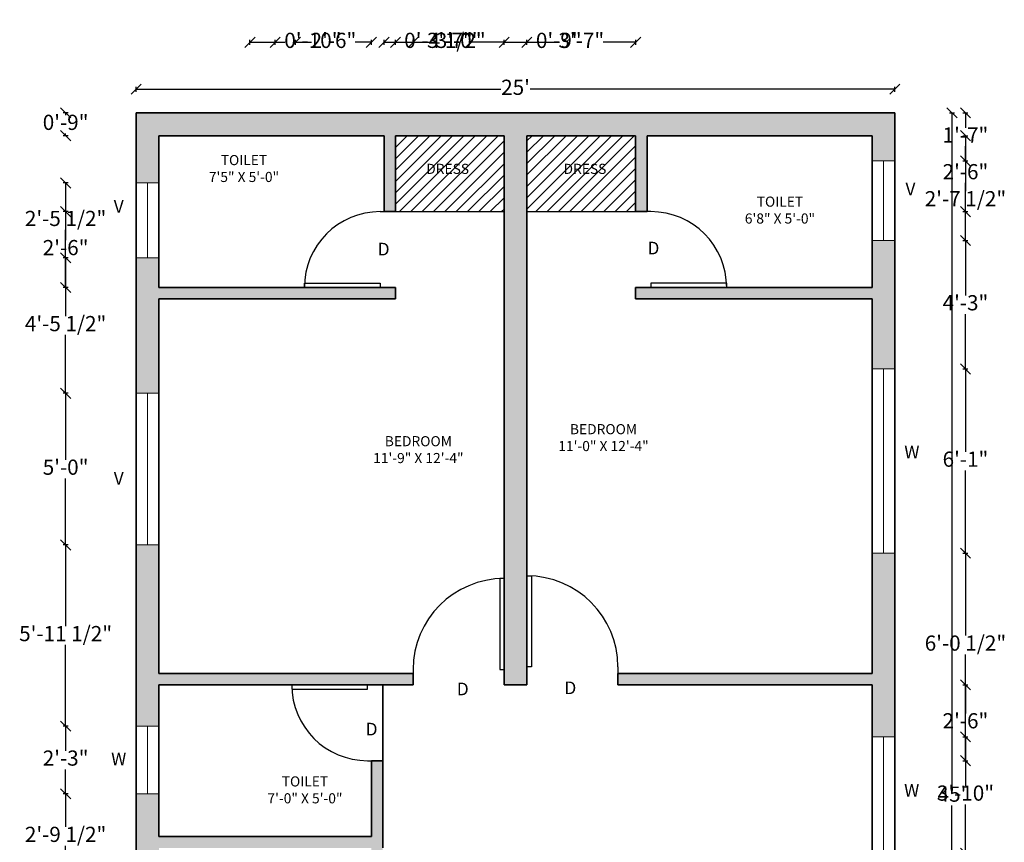
# Model space of a CAD drawing. Units: inches. Extents: x 2633 to 3023, y 679 to 1292.
# Tile 2 of 2: x 2633 to 3023, y 967 to 1292. Entities that reach past the tile are written whole.
import ezdxf

# ---------------------------------------------------------------- set-up
doc = ezdxf.new("R2010")
doc.units = ezdxf.units.IN
for name, color, linetype, lineweight in [('A-ANNO-DIMS', 2, 'Continuous', 18), ('A-ANNO-TEXT', 7, 'Continuous', 18), ('A-AREA-IDEN', 7, 'Continuous', 18), ('A-DOOR', 4, 'Continuous', 25), ('A-FURN', 8, 'Continuous', 25), ('A-FURN-PATT', 8, 'Continuous', 13), ('A-GLAZ', 1, 'Continuous', 18), ('A-WALL', 7, 'Continuous', 35), ('A-WALL-PATT', 5, 'Continuous', 13)]:
    doc.layers.add(name, color=color, linetype=linetype, lineweight=lineweight)
doc.styles.get("Standard").update_dxf_attribs({"font": 'arial.ttf'})
doc.dimstyles.new('ISO-25', dxfattribs={"dimtxt": 6, "dimasz": 4, "dimexe": 1, "dimexo": 1, "dimtad": 0, "dimtih": 1, "dimtoh": 1, "dimlunit": 3, "dimtxsty": 'Standard', "dimblk": 'OBLIQUE', "dimcen": 2.5, "dimadec": 0, "dimazin": 0, "dimtfac": 1, "dimtmove": 0, "dimatfit": 3, "dimfxl": 1, "dimfxlon": 1, "dimarcsym": 0})

# ---------------------------------------------------------------- blocks, each defined once
blk = doc.blocks.new('*U3')
for p, q in [((0, 0), (0, -6)), ((30, 0), (30, -6))]:
    blk.add_line(p, q)
blk.add_lwpolyline([(0, 0), (0, 30), (1.75, 30), (1.75, 0)], close=True)
blk.add_arc((0, 0), 30, 0, 90)
blk = doc.blocks.new('*U9')
for p, q in [((0, 0), (0, -6)), ((-36, 0), (-36, -6))]:
    blk.add_line(p, q)
blk.add_lwpolyline([(0, 0), (0, 36), (-1.75, 36), (-1.75, 0)], close=True)
blk.add_arc((0, 0), 36, 90, 180)
blk = doc.blocks.new('*U10')
for p, q in [((0, 0), (0, 6)), ((30, 0), (30, 6))]:
    blk.add_line(p, q)
blk.add_lwpolyline([(0, 0), (0, -30), (1.75, -30), (1.75, 0)], close=True)
blk.add_arc((0, 0), 30, 270, 0)
blk = doc.blocks.new('*U8')
for p, q in [((0, 0), (0, -6)), ((36, 0), (36, -6))]:
    blk.add_line(p, q)
blk.add_lwpolyline([(0, 0), (0, 36), (1.75, 36), (1.75, 0)], close=True)
blk.add_arc((0, 0), 36, 0, 90)
blk = doc.blocks.new('*U7')
for p, q in [((-30, 0), (-30, -6)), ((0, 0), (0, -6))]:
    blk.add_line(p, q)
blk.add_lwpolyline([(0, 0), (0, 30), (-1.75, 30), (-1.75, 0)], close=True)
blk.add_arc((0, 0), 30, 90, 180)
blk = doc.blocks.new('_Oblique')
at = {"color": 0, "linetype": 'ByBlock', "lineweight": -2}
blk.add_line((-0.5, -0.5), (0.5, 0.5), dxfattribs=at)
blk = doc.blocks.new('*D11')
at = {"layer": 'A-ANNO-DIMS', "color": 0, "lineweight": -2, "transparency": 16777216}
for p, q in [((2679.35, 1263.76), (2679.35, 1265.76)), ((2979.35, 1263.76), (2979.35, 1265.76)), ((2679.35, 1264.76), (2823.58, 1264.76)), ((2979.35, 1264.76), (2835.11, 1264.76))]:
    blk.add_line(p, q, dxfattribs=at)
at = {"layer": 'Defpoints', "color": 0, "transparency": 16777216}
for p in [(2979.35, 1264.76), (2679.35, 1255.4), (2979.35, 1255.4)]:
    blk.add_point(p, dxfattribs=at)
at = {"layer": 'A-ANNO-DIMS', "color": 0, "lineweight": -2, "transparency": 16777216, "xscale": 4, "yscale": 4, "zscale": 4, "rotation": 180}
blk.add_blockref('_Oblique', (2679.35, 1264.76), dxfattribs=at)
at = {"layer": 'A-ANNO-DIMS', "color": 0, "lineweight": -2, "transparency": 16777216, "xscale": 4, "yscale": 4, "zscale": 4}
blk.add_blockref('_Oblique', (2979.35, 1264.76), dxfattribs=at)
at = {"layer": 'A-ANNO-DIMS', "color": 0, "transparency": 16777216, "insert": (2829.35, 1264.76), "char_height": 6, "attachment_point": 5}
blk.add_mtext("25'", dxfattribs=at)
blk = doc.blocks.new('*D12')
at = {"layer": 'A-ANNO-DIMS', "color": 0, "lineweight": -2, "transparency": 16777216}
for p, q in [((3000.92, 1255.4), (3002.92, 1255.4)), ((3001.92, 1255.4), (3001.92, 989.07)), ((3001.92, 715.4), (3001.92, 981.72)), ((3000.92, 715.4), (3002.92, 715.4))]:
    blk.add_line(p, q, dxfattribs=at)
at = {"layer": 'Defpoints', "color": 0, "transparency": 16777216}
for p in [(2979.35, 1255.4), (2979.35, 715.4), (3001.92, 715.4)]:
    blk.add_point(p, dxfattribs=at)
at = {"layer": 'A-ANNO-DIMS', "color": 0, "lineweight": -2, "transparency": 16777216, "xscale": 4, "yscale": 4, "zscale": 4}
for p, rotation in [((3001.92, 1255.4), 90), ((3001.92, 715.4), 270)]:
    blk.add_blockref('_Oblique', p, dxfattribs=dict(at, rotation=rotation))
at = {"layer": 'A-ANNO-DIMS', "color": 0, "transparency": 16777216, "insert": (3001.92, 985.4), "char_height": 6, "attachment_point": 5}
blk.add_mtext("45'", dxfattribs=at)
blk = doc.blocks.new('*D13')
at = {"layer": 'A-ANNO-DIMS', "color": 0, "lineweight": -2, "transparency": 16777216}
for p, q in [((2777.35, 1282.3), (2777.35, 1284.3)), ((2777.35, 1283.3), (2781.85, 1283.3)), ((2781.85, 1282.3), (2781.85, 1284.3)), ((2781.85, 1283.3), (2785.85, 1283.3))]:
    blk.add_line(p, q, dxfattribs=at)
at = {"layer": 'Defpoints', "color": 0, "transparency": 16777216}
for p in [(2781.85, 1283.3), (2777.35, 1246.4), (2781.85, 1246.4)]:
    blk.add_point(p, dxfattribs=at)
at = {"layer": 'A-ANNO-DIMS', "color": 0, "lineweight": -2, "transparency": 16777216, "xscale": 4, "yscale": 4, "zscale": 4, "rotation": 180}
blk.add_blockref('_Oblique', (2777.35, 1283.3), dxfattribs=at)
at = {"layer": 'A-ANNO-DIMS', "color": 0, "lineweight": -2, "transparency": 16777216, "xscale": 4, "yscale": 4, "zscale": 4}
blk.add_blockref('_Oblique', (2781.85, 1283.3), dxfattribs=at)
at = {"layer": 'A-ANNO-DIMS', "color": 0, "transparency": 16777216, "insert": (2801.44, 1283.3), "char_height": 6, "attachment_point": 5}
blk.add_mtext('0\'-4 1/2"', dxfattribs=at)
blk = doc.blocks.new('*D14')
at = {"layer": 'A-ANNO-DIMS', "color": 0, "lineweight": -2, "transparency": 16777216}
for p, q in [((2781.85, 1282.3), (2781.85, 1284.3)), ((2781.85, 1283.3), (2794.75, 1283.3)), ((2824.85, 1283.3), (2811.94, 1283.3)), ((2824.85, 1282.3), (2824.85, 1284.3))]:
    blk.add_line(p, q, dxfattribs=at)
at = {"layer": 'Defpoints', "color": 0, "transparency": 16777216}
for p in [(2824.85, 1283.3), (2781.85, 1246.4), (2824.85, 1246.4)]:
    blk.add_point(p, dxfattribs=at)
at = {"layer": 'A-ANNO-DIMS', "color": 0, "lineweight": -2, "transparency": 16777216, "xscale": 4, "yscale": 4, "zscale": 4, "rotation": 180}
blk.add_blockref('_Oblique', (2781.85, 1283.3), dxfattribs=at)
at = {"layer": 'A-ANNO-DIMS', "color": 0, "lineweight": -2, "transparency": 16777216, "xscale": 4, "yscale": 4, "zscale": 4}
blk.add_blockref('_Oblique', (2824.85, 1283.3), dxfattribs=at)
at = {"layer": 'A-ANNO-DIMS', "color": 0, "transparency": 16777216, "insert": (2803.35, 1283.3), "char_height": 6, "attachment_point": 5}
blk.add_mtext('3\'-7"', dxfattribs=at)
blk = doc.blocks.new('*D15')
at = {"layer": 'A-ANNO-DIMS', "color": 0, "lineweight": -2, "transparency": 16777216}
for p, q in [((2824.85, 1282.3), (2824.85, 1284.3)), ((2824.85, 1283.3), (2833.85, 1283.3)), ((2833.85, 1282.3), (2833.85, 1284.3)), ((2833.85, 1283.3), (2837.85, 1283.3))]:
    blk.add_line(p, q, dxfattribs=at)
at = {"layer": 'Defpoints', "color": 0, "transparency": 16777216}
for p in [(2833.85, 1283.3), (2824.85, 1246.4), (2833.85, 1246.4)]:
    blk.add_point(p, dxfattribs=at)
at = {"layer": 'A-ANNO-DIMS', "color": 0, "lineweight": -2, "transparency": 16777216, "xscale": 4, "yscale": 4, "zscale": 4, "rotation": 180}
blk.add_blockref('_Oblique', (2824.85, 1283.3), dxfattribs=at)
at = {"layer": 'A-ANNO-DIMS', "color": 0, "lineweight": -2, "transparency": 16777216, "xscale": 4, "yscale": 4, "zscale": 4}
blk.add_blockref('_Oblique', (2833.85, 1283.3), dxfattribs=at)
at = {"layer": 'A-ANNO-DIMS', "color": 0, "transparency": 16777216, "insert": (2846.45, 1283.3), "char_height": 6, "attachment_point": 5}
blk.add_mtext('0\'-9"', dxfattribs=at)
blk = doc.blocks.new('*D16')
at = {"layer": 'A-ANNO-DIMS', "color": 0, "lineweight": -2, "transparency": 16777216}
for p, q in [((3006.25, 1246.4), (3008.25, 1246.4)), ((3007.25, 1246.4), (3007.25, 1235.08)), ((3007.25, 1216.4), (3007.25, 1227.71)), ((3006.25, 1216.4), (3008.25, 1216.4))]:
    blk.add_line(p, q, dxfattribs=at)
at = {"layer": 'Defpoints', "color": 0, "transparency": 16777216}
for p in [(2833.85, 1246.4), (3007.25, 1246.4), (2833.85, 1216.4)]:
    blk.add_point(p, dxfattribs=at)
at = {"layer": 'A-ANNO-DIMS', "color": 0, "lineweight": -2, "transparency": 16777216, "xscale": 4, "yscale": 4, "zscale": 4}
for p, rotation in [((3007.25, 1246.4), 90), ((3007.25, 1216.4), 270)]:
    blk.add_blockref('_Oblique', p, dxfattribs=dict(at, rotation=rotation))
at = {"layer": 'A-ANNO-DIMS', "color": 0, "transparency": 16777216, "insert": (3007.25, 1231.4), "char_height": 6, "attachment_point": 5}
blk.add_mtext('2\'-6"', dxfattribs=at)
blk = doc.blocks.new('*D17')
at = {"layer": 'A-ANNO-DIMS', "color": 0, "lineweight": -2, "transparency": 16777216}
for p, q in [((2833.85, 1282.3), (2833.85, 1284.3)), ((2833.85, 1283.3), (2846.75, 1283.3)), ((2876.85, 1283.3), (2863.94, 1283.3)), ((2876.85, 1282.3), (2876.85, 1284.3))]:
    blk.add_line(p, q, dxfattribs=at)
at = {"layer": 'Defpoints', "color": 0, "transparency": 16777216}
for p in [(2876.85, 1283.3), (2833.85, 1246.4), (2876.85, 1246.4)]:
    blk.add_point(p, dxfattribs=at)
at = {"layer": 'A-ANNO-DIMS', "color": 0, "lineweight": -2, "transparency": 16777216, "xscale": 4, "yscale": 4, "zscale": 4, "rotation": 180}
blk.add_blockref('_Oblique', (2833.85, 1283.3), dxfattribs=at)
at = {"layer": 'A-ANNO-DIMS', "color": 0, "lineweight": -2, "transparency": 16777216, "xscale": 4, "yscale": 4, "zscale": 4}
blk.add_blockref('_Oblique', (2876.85, 1283.3), dxfattribs=at)
at = {"layer": 'A-ANNO-DIMS', "color": 0, "transparency": 16777216, "insert": (2855.35, 1283.3), "char_height": 6, "attachment_point": 5}
blk.add_mtext('3\'-7"', dxfattribs=at)
blk = doc.blocks.new('*D20')
at = {"layer": 'A-ANNO-DIMS', "color": 0, "lineweight": -2, "transparency": 16777216}
for p, q in [((2724.35, 1282.3), (2724.35, 1284.3)), ((2724.35, 1283.3), (2734.3, 1283.3)), ((2734.3, 1282.3), (2734.3, 1284.3)), ((2734.3, 1283.3), (2738.3, 1283.3))]:
    blk.add_line(p, q, dxfattribs=at)
at = {"layer": 'Defpoints', "color": 0, "transparency": 16777216}
for p in [(2734.3, 1283.3), (2724.35, 724.4), (2734.3, 724.4)]:
    blk.add_point(p, dxfattribs=at)
at = {"layer": 'A-ANNO-DIMS', "color": 0, "lineweight": -2, "transparency": 16777216, "xscale": 4, "yscale": 4, "zscale": 4, "rotation": 180}
blk.add_blockref('_Oblique', (2724.35, 1283.3), dxfattribs=at)
at = {"layer": 'A-ANNO-DIMS', "color": 0, "lineweight": -2, "transparency": 16777216, "xscale": 4, "yscale": 4, "zscale": 4}
blk.add_blockref('_Oblique', (2734.3, 1283.3), dxfattribs=at)
at = {"layer": 'A-ANNO-DIMS', "color": 0, "transparency": 16777216, "insert": (2749.23, 1283.3), "char_height": 6, "attachment_point": 5}
blk.add_mtext('0\'-10"', dxfattribs=at)
blk = doc.blocks.new('*D23')
at = {"layer": 'A-ANNO-DIMS', "color": 0, "lineweight": -2, "transparency": 16777216}
for p, q in [((2788.85, 1282.3), (2788.85, 1284.3)), ((2788.85, 1283.3), (2798.25, 1283.3)), ((2824.85, 1283.3), (2815.44, 1283.3)), ((2824.85, 1282.3), (2824.85, 1284.3))]:
    blk.add_line(p, q, dxfattribs=at)
at = {"layer": 'Defpoints', "color": 0, "transparency": 16777216}
for p in [(2824.85, 1283.3), (2788.85, 1033.9), (2824.85, 1033.65)]:
    blk.add_point(p, dxfattribs=at)
at = {"layer": 'A-ANNO-DIMS', "color": 0, "lineweight": -2, "transparency": 16777216, "xscale": 4, "yscale": 4, "zscale": 4, "rotation": 180}
blk.add_blockref('_Oblique', (2788.85, 1283.3), dxfattribs=at)
at = {"layer": 'A-ANNO-DIMS', "color": 0, "lineweight": -2, "transparency": 16777216, "xscale": 4, "yscale": 4, "zscale": 4}
blk.add_blockref('_Oblique', (2824.85, 1283.3), dxfattribs=at)
at = {"layer": 'A-ANNO-DIMS', "color": 0, "transparency": 16777216, "insert": (2806.85, 1283.3), "char_height": 6, "attachment_point": 5}
blk.add_mtext('3\'-0"', dxfattribs=at)
blk = doc.blocks.new('*D25')
at = {"layer": 'A-ANNO-DIMS', "color": 0, "lineweight": -2, "transparency": 16777216}
for p, q in [((2742.35, 1282.3), (2742.35, 1284.3)), ((2742.35, 1283.3), (2748.7, 1283.3)), ((2772.35, 1283.3), (2766, 1283.3)), ((2772.35, 1282.3), (2772.35, 1284.3))]:
    blk.add_line(p, q, dxfattribs=at)
at = {"layer": 'Defpoints', "color": 0, "transparency": 16777216}
for p in [(2772.35, 1283.3), (2742.35, 904.9), (2772.35, 904.65)]:
    blk.add_point(p, dxfattribs=at)
at = {"layer": 'A-ANNO-DIMS', "color": 0, "lineweight": -2, "transparency": 16777216, "xscale": 4, "yscale": 4, "zscale": 4, "rotation": 180}
blk.add_blockref('_Oblique', (2742.35, 1283.3), dxfattribs=at)
at = {"layer": 'A-ANNO-DIMS', "color": 0, "lineweight": -2, "transparency": 16777216, "xscale": 4, "yscale": 4, "zscale": 4}
blk.add_blockref('_Oblique', (2772.35, 1283.3), dxfattribs=at)
at = {"layer": 'A-ANNO-DIMS', "color": 0, "transparency": 16777216, "insert": (2757.35, 1283.3), "char_height": 6, "attachment_point": 5}
blk.add_mtext('2\'-6"', dxfattribs=at)
blk = doc.blocks.new('*D26')
at = {"layer": 'A-ANNO-DIMS', "color": 0, "lineweight": -2, "transparency": 16777216}
for p, q in [((2652.45, 1216.4), (2650.45, 1216.4)), ((2651.45, 1216.4), (2651.45, 1205.08)), ((2651.45, 1186.4), (2651.45, 1197.71)), ((2652.45, 1186.4), (2650.45, 1186.4))]:
    blk.add_line(p, q, dxfattribs=at)
at = {"layer": 'Defpoints', "color": 0, "transparency": 16777216}
for p in [(2777.35, 1216.4), (2651.45, 1186.4), (2777.6, 1186.4)]:
    blk.add_point(p, dxfattribs=at)
at = {"layer": 'A-ANNO-DIMS', "color": 0, "lineweight": -2, "transparency": 16777216, "xscale": 4, "yscale": 4, "zscale": 4}
for p, rotation in [((2651.45, 1216.4), 90), ((2651.45, 1186.4), 270)]:
    blk.add_blockref('_Oblique', p, dxfattribs=dict(at, rotation=rotation))
at = {"layer": 'A-ANNO-DIMS', "color": 0, "transparency": 16777216, "insert": (2651.45, 1201.4), "char_height": 6, "attachment_point": 5}
blk.add_mtext('2\'-6"', dxfattribs=at)
blk = doc.blocks.new('*D27')
at = {"layer": 'A-ANNO-DIMS', "color": 0, "lineweight": -2, "transparency": 16777216}
for p, q in [((3006.25, 1029.4), (3008.25, 1029.4)), ((3007.25, 1029.4), (3007.25, 1018.08)), ((3007.25, 999.4), (3007.25, 1010.71)), ((3006.25, 999.4), (3008.25, 999.4))]:
    blk.add_line(p, q, dxfattribs=at)
at = {"layer": 'Defpoints', "color": 0, "transparency": 16777216}
for p in [(2776.85, 1029.4), (3007.25, 1029.4), (2776.85, 999.4)]:
    blk.add_point(p, dxfattribs=at)
at = {"layer": 'A-ANNO-DIMS', "color": 0, "lineweight": -2, "transparency": 16777216, "xscale": 4, "yscale": 4, "zscale": 4}
for p, rotation in [((3007.25, 1029.4), 90), ((3007.25, 999.4), 270)]:
    blk.add_blockref('_Oblique', p, dxfattribs=dict(at, rotation=rotation))
at = {"layer": 'A-ANNO-DIMS', "color": 0, "transparency": 16777216, "insert": (3007.25, 1014.4), "char_height": 6, "attachment_point": 5}
blk.add_mtext('2\'-6"', dxfattribs=at)
blk = doc.blocks.new('*D28')
at = {"layer": 'A-ANNO-DIMS', "color": 0, "lineweight": -2, "transparency": 16777216}
for p, q in [((2652.45, 1255.4), (2650.45, 1255.4)), ((2651.45, 1255.4), (2651.45, 1254.58)), ((2652.45, 1246.4), (2650.45, 1246.4)), ((2651.45, 1246.4), (2651.45, 1247.21))]:
    blk.add_line(p, q, dxfattribs=at)
at = {"layer": 'Defpoints', "color": 0, "transparency": 16777216}
for p in [(2679.35, 1255.4), (2651.45, 1246.4), (2688.35, 1246.4)]:
    blk.add_point(p, dxfattribs=at)
at = {"layer": 'A-ANNO-DIMS', "color": 0, "lineweight": -2, "transparency": 16777216, "xscale": 4, "yscale": 4, "zscale": 4}
for p, rotation in [((2651.45, 1255.4), 90), ((2651.45, 1246.4), 270)]:
    blk.add_blockref('_Oblique', p, dxfattribs=dict(at, rotation=rotation))
at = {"layer": 'A-ANNO-DIMS', "color": 0, "transparency": 16777216, "insert": (2651.45, 1250.9), "char_height": 6, "attachment_point": 5}
blk.add_mtext('0\'-9"', dxfattribs=at)
blk = doc.blocks.new('*D33')
at = {"layer": 'A-ANNO-DIMS', "color": 0, "lineweight": -2, "transparency": 16777216}
for p, q in [((2652.45, 986.26), (2650.45, 986.26)), ((2651.45, 986.26), (2651.45, 973.23)), ((2651.45, 952.74), (2651.45, 965.77)), ((2652.45, 952.74), (2650.45, 952.74))]:
    blk.add_line(p, q, dxfattribs=at)
at = {"layer": 'Defpoints', "color": 0, "transparency": 16777216}
for p in [(2651.45, 986.26), (2679.35, 986.26), (2679.35, 952.74)]:
    blk.add_point(p, dxfattribs=at)
at = {"layer": 'A-ANNO-DIMS', "color": 0, "lineweight": -2, "transparency": 16777216, "xscale": 4, "yscale": 4, "zscale": 4}
for p, rotation in [((2651.45, 986.26), 90), ((2651.45, 952.74), 270)]:
    blk.add_blockref('_Oblique', p, dxfattribs=dict(at, rotation=rotation))
at = {"layer": 'A-ANNO-DIMS', "color": 0, "transparency": 16777216, "insert": (2651.45, 969.5), "char_height": 6, "attachment_point": 5}
blk.add_mtext('2\'-9 1/2"', dxfattribs=at)
blk = doc.blocks.new('*D34')
at = {"layer": 'A-ANNO-DIMS', "color": 0, "lineweight": -2, "transparency": 16777216}
for p, q in [((2652.45, 1013.04), (2650.45, 1013.04)), ((2651.45, 1013.04), (2651.45, 1003.34)), ((2651.45, 986.26), (2651.45, 995.96)), ((2652.45, 986.26), (2650.45, 986.26))]:
    blk.add_line(p, q, dxfattribs=at)
at = {"layer": 'Defpoints', "color": 0, "transparency": 16777216}
for p in [(2651.45, 1013.04), (2679.35, 1013.04), (2679.35, 986.26)]:
    blk.add_point(p, dxfattribs=at)
at = {"layer": 'A-ANNO-DIMS', "color": 0, "lineweight": -2, "transparency": 16777216, "xscale": 4, "yscale": 4, "zscale": 4}
for p, rotation in [((2651.45, 1013.04), 90), ((2651.45, 986.26), 270)]:
    blk.add_blockref('_Oblique', p, dxfattribs=dict(at, rotation=rotation))
at = {"layer": 'A-ANNO-DIMS', "color": 0, "transparency": 16777216, "insert": (2651.45, 999.65), "char_height": 6, "attachment_point": 5}
blk.add_mtext('2\'-3"', dxfattribs=at)
blk = doc.blocks.new('*D35')
at = {"layer": 'A-ANNO-DIMS', "color": 0, "lineweight": -2, "transparency": 16777216}
for p, q in [((2652.45, 1084.66), (2650.45, 1084.66)), ((2651.45, 1084.66), (2651.45, 1052.58)), ((2651.45, 1013.04), (2651.45, 1045.12)), ((2652.45, 1013.04), (2650.45, 1013.04))]:
    blk.add_line(p, q, dxfattribs=at)
at = {"layer": 'Defpoints', "color": 0, "transparency": 16777216}
for p in [(2651.45, 1084.66), (2679.35, 1084.66), (2679.35, 1013.04)]:
    blk.add_point(p, dxfattribs=at)
at = {"layer": 'A-ANNO-DIMS', "color": 0, "lineweight": -2, "transparency": 16777216, "xscale": 4, "yscale": 4, "zscale": 4}
for p, rotation in [((2651.45, 1084.66), 90), ((2651.45, 1013.04), 270)]:
    blk.add_blockref('_Oblique', p, dxfattribs=dict(at, rotation=rotation))
at = {"layer": 'A-ANNO-DIMS', "color": 0, "transparency": 16777216, "insert": (2651.45, 1048.85), "char_height": 6, "attachment_point": 5}
blk.add_mtext('5\'-11 1/2"', dxfattribs=at)
blk = doc.blocks.new('*D36')
at = {"layer": 'A-ANNO-DIMS', "color": 0, "lineweight": -2, "transparency": 16777216}
for p, q in [((2652.45, 1144.59), (2650.45, 1144.59)), ((2651.45, 1144.59), (2651.45, 1118.31)), ((2651.45, 1084.66), (2651.45, 1110.94)), ((2652.45, 1084.66), (2650.45, 1084.66))]:
    blk.add_line(p, q, dxfattribs=at)
at = {"layer": 'Defpoints', "color": 0, "transparency": 16777216}
for p in [(2651.45, 1144.59), (2679.35, 1144.59), (2679.35, 1084.66)]:
    blk.add_point(p, dxfattribs=at)
at = {"layer": 'A-ANNO-DIMS', "color": 0, "lineweight": -2, "transparency": 16777216, "xscale": 4, "yscale": 4, "zscale": 4}
for p, rotation in [((2651.45, 1144.59), 90), ((2651.45, 1084.66), 270)]:
    blk.add_blockref('_Oblique', p, dxfattribs=dict(at, rotation=rotation))
at = {"layer": 'A-ANNO-DIMS', "color": 0, "transparency": 16777216, "insert": (2651.45, 1114.62), "char_height": 6, "attachment_point": 5}
blk.add_mtext('5\'-0"', dxfattribs=at)
blk = doc.blocks.new('*D37')
at = {"layer": 'A-ANNO-DIMS', "color": 0, "lineweight": -2, "transparency": 16777216}
for p, q in [((2652.45, 1198.14), (2650.45, 1198.14)), ((2651.45, 1198.14), (2651.45, 1175.09)), ((2651.45, 1144.59), (2651.45, 1167.64)), ((2652.45, 1144.59), (2650.45, 1144.59))]:
    blk.add_line(p, q, dxfattribs=at)
at = {"layer": 'Defpoints', "color": 0, "transparency": 16777216}
for p in [(2651.45, 1198.14), (2679.35, 1198.14), (2679.35, 1144.59)]:
    blk.add_point(p, dxfattribs=at)
at = {"layer": 'A-ANNO-DIMS', "color": 0, "lineweight": -2, "transparency": 16777216, "xscale": 4, "yscale": 4, "zscale": 4}
for p, rotation in [((2651.45, 1198.14), 90), ((2651.45, 1144.59), 270)]:
    blk.add_blockref('_Oblique', p, dxfattribs=dict(at, rotation=rotation))
at = {"layer": 'A-ANNO-DIMS', "color": 0, "transparency": 16777216, "insert": (2651.45, 1171.36), "char_height": 6, "attachment_point": 5}
blk.add_mtext('4\'-5 1/2"', dxfattribs=at)
blk = doc.blocks.new('*D38')
at = {"layer": 'A-ANNO-DIMS', "color": 0, "lineweight": -2, "transparency": 16777216}
for p, q in [((2652.45, 1227.71), (2650.45, 1227.71)), ((2651.45, 1227.71), (2651.45, 1216.65)), ((2651.45, 1198.14), (2651.45, 1209.2)), ((2652.45, 1198.14), (2650.45, 1198.14))]:
    blk.add_line(p, q, dxfattribs=at)
at = {"layer": 'Defpoints', "color": 0, "transparency": 16777216}
for p in [(2651.45, 1227.71), (2679.35, 1227.71), (2679.35, 1198.14)]:
    blk.add_point(p, dxfattribs=at)
at = {"layer": 'A-ANNO-DIMS', "color": 0, "lineweight": -2, "transparency": 16777216, "xscale": 4, "yscale": 4, "zscale": 4}
for p, rotation in [((2651.45, 1227.71), 90), ((2651.45, 1198.14), 270)]:
    blk.add_blockref('_Oblique', p, dxfattribs=dict(at, rotation=rotation))
at = {"layer": 'A-ANNO-DIMS', "color": 0, "transparency": 16777216, "insert": (2651.45, 1212.92), "char_height": 6, "attachment_point": 5}
blk.add_mtext('2\'-5 1/2"', dxfattribs=at)
blk = doc.blocks.new('*D42')
at = {"layer": 'A-ANNO-DIMS', "color": 0, "lineweight": -2, "transparency": 16777216}
for p, q in [((3006.25, 1008.83), (3008.25, 1008.83)), ((3007.25, 1008.83), (3007.25, 989.5)), ((3007.25, 962.79), (3007.25, 982.12)), ((3006.25, 962.79), (3008.25, 962.79))]:
    blk.add_line(p, q, dxfattribs=at)
at = {"layer": 'Defpoints', "color": 0, "transparency": 16777216}
for p in [(2979.35, 1008.83), (3007.25, 1008.83), (2979.35, 962.79)]:
    blk.add_point(p, dxfattribs=at)
at = {"layer": 'A-ANNO-DIMS', "color": 0, "lineweight": -2, "transparency": 16777216, "xscale": 4, "yscale": 4, "zscale": 4}
for p, rotation in [((3007.25, 1008.83), 90), ((3007.25, 962.79), 270)]:
    blk.add_blockref('_Oblique', p, dxfattribs=dict(at, rotation=rotation))
at = {"layer": 'A-ANNO-DIMS', "color": 0, "transparency": 16777216, "insert": (3007.25, 985.81), "char_height": 6, "attachment_point": 5}
blk.add_mtext('3\'-10"', dxfattribs=at)
blk = doc.blocks.new('*D43')
at = {"layer": 'A-ANNO-DIMS', "color": 0, "lineweight": -2, "transparency": 16777216}
for p, q in [((3006.25, 1081.38), (3008.25, 1081.38)), ((3007.25, 1081.38), (3007.25, 1048.83)), ((3007.25, 1008.83), (3007.25, 1041.38)), ((3006.25, 1008.83), (3008.25, 1008.83))]:
    blk.add_line(p, q, dxfattribs=at)
at = {"layer": 'Defpoints', "color": 0, "transparency": 16777216}
for p in [(2979.35, 1081.38), (3007.25, 1081.38), (2979.35, 1008.83)]:
    blk.add_point(p, dxfattribs=at)
at = {"layer": 'A-ANNO-DIMS', "color": 0, "lineweight": -2, "transparency": 16777216, "xscale": 4, "yscale": 4, "zscale": 4}
for p, rotation in [((3007.25, 1081.38), 90), ((3007.25, 1008.83), 270)]:
    blk.add_blockref('_Oblique', p, dxfattribs=dict(at, rotation=rotation))
at = {"layer": 'A-ANNO-DIMS', "color": 0, "transparency": 16777216, "insert": (3007.25, 1045.1), "char_height": 6, "attachment_point": 5}
blk.add_mtext('6\'-0 1/2"', dxfattribs=at)
blk = doc.blocks.new('*D44')
at = {"layer": 'A-ANNO-DIMS', "color": 0, "lineweight": -2, "transparency": 16777216}
for p, q in [((3006.25, 1154.2), (3008.25, 1154.2)), ((3007.25, 1154.2), (3007.25, 1121.48)), ((3007.25, 1081.38), (3007.25, 1114.1)), ((3006.25, 1081.38), (3008.25, 1081.38))]:
    blk.add_line(p, q, dxfattribs=at)
at = {"layer": 'Defpoints', "color": 0, "transparency": 16777216}
for p in [(2979.35, 1154.2), (3007.25, 1154.2), (2979.35, 1081.38)]:
    blk.add_point(p, dxfattribs=at)
at = {"layer": 'A-ANNO-DIMS', "color": 0, "lineweight": -2, "transparency": 16777216, "xscale": 4, "yscale": 4, "zscale": 4}
for p, rotation in [((3007.25, 1154.2), 90), ((3007.25, 1081.38), 270)]:
    blk.add_blockref('_Oblique', p, dxfattribs=dict(at, rotation=rotation))
at = {"layer": 'A-ANNO-DIMS', "color": 0, "transparency": 16777216, "insert": (3007.25, 1117.79), "char_height": 6, "attachment_point": 5}
blk.add_mtext('6\'-1"', dxfattribs=at)
blk = doc.blocks.new('*D45')
at = {"layer": 'A-ANNO-DIMS', "color": 0, "lineweight": -2, "transparency": 16777216}
for p, q in [((3006.25, 1205.01), (3008.25, 1205.01)), ((3007.25, 1205.01), (3007.25, 1183.29)), ((3007.25, 1154.2), (3007.25, 1175.91)), ((3006.25, 1154.2), (3008.25, 1154.2))]:
    blk.add_line(p, q, dxfattribs=at)
at = {"layer": 'Defpoints', "color": 0, "transparency": 16777216}
for p in [(2979.35, 1205.01), (3007.25, 1205.01), (2979.35, 1154.2)]:
    blk.add_point(p, dxfattribs=at)
at = {"layer": 'A-ANNO-DIMS', "color": 0, "lineweight": -2, "transparency": 16777216, "xscale": 4, "yscale": 4, "zscale": 4}
for p, rotation in [((3007.25, 1205.01), 90), ((3007.25, 1154.2), 270)]:
    blk.add_blockref('_Oblique', p, dxfattribs=dict(at, rotation=rotation))
at = {"layer": 'A-ANNO-DIMS', "color": 0, "transparency": 16777216, "insert": (3007.25, 1179.6), "char_height": 6, "attachment_point": 5}
blk.add_mtext('4\'-3"', dxfattribs=at)
blk = doc.blocks.new('*D46')
at = {"layer": 'A-ANNO-DIMS', "color": 0, "lineweight": -2, "transparency": 16777216}
for p, q in [((3006.25, 1236.41), (3008.25, 1236.41)), ((3007.25, 1236.41), (3007.25, 1224.44)), ((3007.25, 1205.01), (3007.25, 1216.98)), ((3006.25, 1205.01), (3008.25, 1205.01))]:
    blk.add_line(p, q, dxfattribs=at)
at = {"layer": 'Defpoints', "color": 0, "transparency": 16777216}
for p in [(2979.35, 1236.41), (3007.25, 1236.41), (2979.35, 1205.01)]:
    blk.add_point(p, dxfattribs=at)
at = {"layer": 'A-ANNO-DIMS', "color": 0, "lineweight": -2, "transparency": 16777216, "xscale": 4, "yscale": 4, "zscale": 4}
for p, rotation in [((3007.25, 1236.41), 90), ((3007.25, 1205.01), 270)]:
    blk.add_blockref('_Oblique', p, dxfattribs=dict(at, rotation=rotation))
at = {"layer": 'A-ANNO-DIMS', "color": 0, "transparency": 16777216, "insert": (3007.25, 1220.71), "char_height": 6, "attachment_point": 5}
blk.add_mtext('2\'-7 1/2"', dxfattribs=at)
blk = doc.blocks.new('*D47')
at = {"layer": 'A-ANNO-DIMS', "color": 0, "lineweight": -2, "transparency": 16777216}
for p, q in [((3006.25, 1255.4), (3008.25, 1255.4)), ((3007.25, 1255.4), (3007.25, 1249.54)), ((3007.25, 1236.41), (3007.25, 1242.27)), ((3006.25, 1236.41), (3008.25, 1236.41))]:
    blk.add_line(p, q, dxfattribs=at)
at = {"layer": 'Defpoints', "color": 0, "transparency": 16777216}
for p in [(2979.35, 1255.4), (3007.25, 1255.4), (2979.35, 1236.41)]:
    blk.add_point(p, dxfattribs=at)
at = {"layer": 'A-ANNO-DIMS', "color": 0, "lineweight": -2, "transparency": 16777216, "xscale": 4, "yscale": 4, "zscale": 4}
for p, rotation in [((3007.25, 1255.4), 90), ((3007.25, 1236.41), 270)]:
    blk.add_blockref('_Oblique', p, dxfattribs=dict(at, rotation=rotation))
at = {"layer": 'A-ANNO-DIMS', "color": 0, "transparency": 16777216, "insert": (3007.25, 1245.9), "char_height": 6, "attachment_point": 5}
blk.add_mtext('1\'-7"', dxfattribs=at)

msp = doc.modelspace()

# ---------------------------------------------------------------- hatches: boundary and pattern name
at = {"layer": 'A-FURN-PATT'}
h = msp.add_hatch(dxfattribs=at)
h.set_pattern_fill('ANSI31', color=256)
h.paths.add_polyline_path([(2824.847, 1246.396), (2781.847, 1246.396), (2781.847, 1216.396), (2824.847, 1216.396)])
h.paths.add_polyline_path([(2876.847, 1246.396), (2833.847, 1246.396), (2833.847, 1216.396), (2876.847, 1216.396)])
h.paths.add_polyline_path([(2791.81, 1229.045), (2813.063, 1229.045), (2813.063, 1237.288), (2791.81, 1237.288)], flags=24)
h.paths.add_polyline_path([(2846.101, 1229.045), (2867.354, 1229.045), (2867.354, 1237.288), (2846.101, 1237.288)], flags=24)
at = {"layer": 'A-WALL-PATT'}
h = msp.add_hatch(color=256, dxfattribs=at)
h.dxf.hatch_style = 1
h.paths.add_polyline_path([(2777.347, 1246.396), (2777.347, 1216.396), (2781.847, 1216.396), (2781.847, 1246.396), (2824.847, 1246.396), (2824.847, 1029.396), (2833.847, 1029.396), (2833.847, 1246.396), (2876.847, 1246.396), (2876.847, 1216.396), (2881.347, 1216.396), (2881.347, 1246.396), (2970.347, 1246.396), (2970.347, 1236.412), (2979.347, 1236.412), (2979.347, 1255.396), (2679.347, 1255.396), (2679.347, 1227.707), (2688.347, 1227.707), (2688.347, 1246.396)])
h.paths.add_polyline_path([(2688.347, 1033.896), (2688.347, 1084.661), (2679.347, 1084.661), (2679.347, 1013.042), (2688.347, 1013.042), (2688.347, 1029.396), (2776.847, 1029.396), (2788.847, 1029.396), (2788.847, 1033.896)])
h.paths.add_polyline_path([(2679.347, 952.735), (2688.347, 952.735), (2688.347, 964.896), (2772.347, 964.896), (2772.347, 900.396), (2776.847, 900.396), (2776.847, 964.896), (2776.847, 999.396), (2772.347, 999.396), (2772.347, 969.396), (2688.347, 969.396), (2688.347, 986.261), (2679.347, 986.261)])
h.paths.add_polyline_path([(2688.347, 1181.896), (2781.847, 1181.896), (2781.847, 1186.396), (2688.347, 1186.396), (2688.347, 1198.143), (2679.347, 1198.143), (2679.347, 1144.586), (2688.347, 1144.586)], flags=17)
h.paths.add_polyline_path([(2688.347, 900.396), (2742.347, 900.396), (2742.347, 904.896), (2688.347, 904.896), (2688.347, 919.665), (2679.347, 919.665), (2679.347, 872.753), (2688.347, 872.753)])
h.paths.add_polyline_path([(2679.347, 715.396), (2841.347, 715.396), (2841.347, 724.396), (2688.347, 724.396), (2688.347, 796.396), (2838.347, 796.396), (2838.347, 804.396), (2829.347, 804.396), (2688.347, 804.396), (2688.347, 838.241), (2679.347, 838.241)])
h.paths.add_polyline_path([(2838.347, 904.896), (2808.847, 904.896), (2808.847, 900.396), (2829.347, 900.396), (2829.347, 852.396), (2838.347, 852.396)])
h.paths.add_polyline_path([(2970.347, 856.396), (2943.46, 856.396), (2943.46, 847.396), (2970.347, 847.396), (2970.347, 715.396), (2979.347, 715.396), (2979.347, 872.317), (2970.347, 872.317)])
h.paths.add_polyline_path([(2979.347, 962.792), (2970.347, 962.792), (2970.347, 911.933), (2979.347, 911.933)])
h.paths.add_polyline_path([(2979.347, 1081.378), (2970.347, 1081.378), (2970.347, 1033.896), (2869.847, 1033.896), (2869.847, 1029.396), (2970.347, 1029.396), (2970.347, 1008.832), (2979.347, 1008.832)])
h.paths.add_polyline_path([(2979.347, 1205.007), (2970.347, 1205.007), (2970.347, 1186.396), (2876.847, 1186.396), (2876.847, 1181.896), (2970.347, 1181.896), (2970.347, 1154.2), (2979.347, 1154.2)], flags=17)
h.paths.add_polyline_path([(2901.589, 847.396), (2901.589, 856.396), (2886.347, 856.396), (2886.347, 847.396)])

# ---------------------------------------------------------------- linework, layer by layer
at = {"layer": 'A-FURN'}
for p, q in [((2781.847, 1216.396), (2824.847, 1216.396)), ((2833.847, 1216.396), (2876.847, 1216.396))]:
    msp.add_line(p, q, dxfattribs=at)
at = {"layer": 'A-GLAZ'}
for p, q in [((2970.347, 1236.412), (2979.347, 1236.412)), ((2974.847, 1236.412), (2974.847, 1205.007)), ((2688.347, 1227.707), (2679.347, 1227.707)), ((2683.847, 1198.143), (2683.847, 1227.707)), ((2970.347, 1205.007), (2979.347, 1205.007)), ((2688.347, 1198.143), (2679.347, 1198.143)), ((2970.347, 1154.2), (2979.347, 1154.2)), ((2974.847, 1154.2), (2974.847, 1081.378)), ((2688.347, 1144.586), (2679.347, 1144.586)), ((2683.847, 1144.586), (2683.847, 1084.661)), ((2688.347, 1084.661), (2679.347, 1084.661)), ((2970.347, 1081.378), (2979.347, 1081.378)), ((2688.347, 1013.042), (2679.347, 1013.042)), ((2683.847, 986.261), (2683.847, 1013.042)), ((2970.347, 1008.832), (2979.347, 1008.832)), ((2974.847, 1008.832), (2974.847, 962.792)), ((2688.347, 986.261), (2679.347, 986.261))]:
    msp.add_line(p, q, dxfattribs=at)
at = {"layer": 'A-WALL'}
for p, q in [((2979.347, 1255.396), (2679.347, 1255.396)), ((2679.347, 1255.396), (2679.347, 715.396)), ((2979.347, 715.396), (2979.347, 1255.396)), ((2688.347, 1246.396), (2688.347, 1186.396)), ((2777.347, 1246.396), (2688.347, 1246.396)), ((2777.347, 1246.396), (2777.347, 1216.396)), ((2781.847, 1246.396), (2781.847, 1216.396)), ((2824.847, 1246.396), (2781.847, 1246.396)), ((2824.847, 1029.396), (2824.847, 1246.396)), ((2876.847, 1246.396), (2833.847, 1246.396)), ((2833.847, 1029.396), (2833.847, 1246.396)), ((2876.847, 1216.396), (2876.847, 1246.396)), ((2970.347, 1246.396), (2881.347, 1246.396)), ((2881.347, 1216.396), (2881.347, 1246.396)), ((2970.347, 1186.396), (2970.347, 1246.396)), ((2777.347, 1216.396), (2781.847, 1216.396)), ((2876.847, 1216.396), (2881.347, 1216.396)), ((2781.847, 1186.396), (2688.347, 1186.396)), ((2781.847, 1186.396), (2781.847, 1181.896)), ((2970.347, 1186.396), (2876.847, 1186.396)), ((2876.847, 1181.896), (2876.847, 1186.396)), ((2688.347, 1181.896), (2688.347, 1033.896)), ((2781.847, 1181.896), (2688.347, 1181.896)), ((2970.347, 1181.896), (2876.847, 1181.896)), ((2970.347, 1033.896), (2970.347, 1181.896)), ((2788.847, 1033.896), (2688.347, 1033.896)), ((2788.847, 1033.896), (2788.847, 1029.396)), ((2970.347, 1033.896), (2869.847, 1033.896)), ((2869.847, 1029.396), (2869.847, 1033.896)), ((2688.347, 1029.396), (2688.347, 969.396)), ((2776.847, 1029.396), (2688.347, 1029.396)), ((2776.847, 1029.396), (2776.847, 964.896)), ((2788.847, 1029.396), (2776.847, 1029.396)), ((2833.847, 1029.396), (2824.847, 1029.396)), ((2970.347, 1029.396), (2869.847, 1029.396)), ((2970.347, 856.396), (2970.347, 1029.396)), ((2772.347, 999.396), (2772.347, 969.396)), ((2772.347, 999.396), (2776.847, 999.396)), ((2772.347, 969.396), (2688.347, 969.396))]:
    msp.add_line(p, q, dxfattribs=at)

# ---------------------------------------------------------------- block references
at = {"layer": 'A-DOOR', "rotation": 90}
for name, p in [('*U3', (2775.847, 1186.396)), ('*U10', (2882.847, 1186.396)), ('*U7', (2770.847, 1029.396))]:
    msp.add_blockref(name, p, dxfattribs=at)
at = {"layer": 'A-DOOR'}
for name, p in [('*U9', (2824.847, 1035.396)), ('*U8', (2833.847, 1036.445))]:
    msp.add_blockref(name, p, dxfattribs=at)

# ---------------------------------------------------------------- texts
at = {"layer": 'A-ANNO-TEXT', "char_height": 5, "attachment_point": 1}
for s, insert in [('\\pxqc;V', (2982.09, 1227.843)), ('\\pxqc;V', (2669.038, 1220.938)), ('\\pxqc;D', (2773.789, 1204.07)), ('\\pxqc;D', (2880.47, 1204.483)), ('\\pxqc;W', (2982.649, 1123.873)), ('\\pxqc;V', (2669.038, 1113.512)), ('\\pxqc;D', (2805.074, 1030.243)), ('\\pxqc;D', (2847.612, 1030.691)), ('\\pxqc;D', (2769.029, 1014.367)), ('\\pxqc;W', (2669.038, 1002.617)), ('\\pxqc;W', (2982.582, 990.184))]:
    msp.add_mtext_dynamic_manual_height_columns(s, width=6.8199, gutter_width=12.5, heights=[0], dxfattribs=dict(at, insert=insert))
at = {"layer": 'A-AREA-IDEN', "char_height": 4, "attachment_point": 1}
for s, width, insert in [('\\pxqc;TOILET\\P7\'5" X 5\'-0"', 33.8072, (2705.067, 1238.761)), ('\\pxqc;DRESS', 33.8072, (2785.603, 1235.298)), ('\\pxqc;DRESS', 33.8072, (2839.894, 1235.298)), ('\\pxqc;TOILET\\P6\'8" X 5\'-0"', 33.8072, (2916.993, 1222.343)), ('\\pxqc;BEDROOM\\P11\'-0" X 12\'-4"', 38.24328, (2845.002, 1132.415)), ('\\pxqc;BEDROOM\\P11\'-9" X 12\'-4"', 41.82244, (2770.008, 1127.669)), ('\\pxqc;TOILET\\P7\'-0" X 5\'-0"', 33.8072, (2729.182, 993.201))]:
    msp.add_mtext_dynamic_manual_height_columns(s, width=width, gutter_width=12.5, heights=[0], dxfattribs=dict(at, insert=insert))

# ---------------------------------------------------------------- dimensions: what is measured, and where the dimension line sits
at = {"layer": 'A-ANNO-DIMS'}
for base, p1, p2, override, picture, middle in [((2781.847, 1283.296), (2777.347, 1246.396), (2781.847, 1246.396), {"dimdec": 1, "dimlfac": 1, "dimrnd": 0, "dimzin": 1, "dimdsep": 46, "dimlunit": 4, "dimfrac": 2}, '*D13', (2801.437, 1283.296)), ((2734.302, 1283.296), (2724.347, 724.396), (2734.302, 724.396), {"dimdec": 1, "dimlfac": 1, "dimrnd": 0, "dimzin": 1, "dimdsep": 46, "dimlunit": 4, "dimfrac": 2}, '*D20', (2749.232, 1283.296)), ((2772.347, 1283.296), (2742.347, 904.896), (2772.347, 904.646), {"dimdec": 1, "dimlfac": 1, "dimrnd": 0, "dimzin": 1, "dimdsep": 46, "dimlunit": 4, "dimfrac": 2}, '*D25', (2757.347, 1283.296)), ((2824.847, 1283.296), (2781.847, 1246.396), (2824.847, 1246.396), {"dimdec": 1, "dimlfac": 1, "dimrnd": 0, "dimzin": 1, "dimdsep": 46, "dimlunit": 4, "dimfrac": 2}, '*D14', (2803.347, 1283.296)), ((2824.847, 1283.296), (2788.847, 1033.896), (2824.847, 1033.646), {"dimdec": 1, "dimlfac": 1, "dimrnd": 0, "dimzin": 1, "dimdsep": 46, "dimlunit": 4, "dimfrac": 2}, '*D23', (2806.847, 1283.296)), ((2833.847, 1283.296), (2824.847, 1246.396), (2833.847, 1246.396), {"dimdec": 1, "dimlfac": 1, "dimrnd": 0, "dimzin": 1, "dimdsep": 46, "dimlunit": 4, "dimfrac": 2}, '*D15', (2846.447, 1283.296)), ((2876.847, 1283.296), (2833.847, 1246.396), (2876.847, 1246.396), {"dimdec": 1, "dimlfac": 1, "dimrnd": 0, "dimzin": 1, "dimdsep": 46, "dimlunit": 4, "dimfrac": 2}, '*D17', (2855.347, 1283.296)), ((2979.347, 1264.762), (2679.347, 1255.396), (2979.347, 1255.396), {"dimclrd": 0, "dimclre": 0, "dimclrt": 0}, '*D11', (2829.347, 1264.762))]:
    dim = msp.add_linear_dim(base=base, p1=p1, p2=p2, dimstyle='ISO-25', override=override, dxfattribs=at)
    dim.commit()
    dim.dimension.update_dxf_attribs({"geometry": picture, "text_midpoint": middle})
for base, p1, p2, override, picture, middle in [((2651.447, 1246.396), (2679.347, 1255.396), (2688.347, 1246.396), {"dimdec": 1, "dimlfac": 1, "dimrnd": 0, "dimzin": 1, "dimdsep": 46, "dimlunit": 4, "dimfrac": 2}, '*D28', (2651.447, 1250.896)), ((3001.916, 715.396), (2979.347, 1255.396), (2979.347, 715.396), {"dimclrd": 0, "dimclre": 0, "dimclrt": 0}, '*D12', (3001.916, 985.396)), ((3007.247, 1255.396), (2979.347, 1236.412), (2979.347, 1255.396), {"dimdec": 1, "dimlfac": 1, "dimrnd": 0, "dimzin": 1, "dimdsep": 46, "dimlunit": 4, "dimfrac": 2}, '*D47', (3007.247, 1245.904)), ((3007.247, 1246.396), (2833.847, 1216.396), (2833.847, 1246.396), {"dimdec": 1, "dimlfac": 1, "dimrnd": 0, "dimzin": 1, "dimdsep": 46, "dimlunit": 4, "dimfrac": 2}, '*D16', (3007.247, 1231.396)), ((3007.247, 1236.412), (2979.347, 1205.007), (2979.347, 1236.412), {"dimdec": 1, "dimlfac": 1, "dimrnd": 0, "dimzin": 1, "dimdsep": 46, "dimlunit": 4, "dimfrac": 2}, '*D46', (3007.247, 1220.709)), ((2651.447, 1227.707), (2679.347, 1198.143), (2679.347, 1227.707), {"dimdec": 1, "dimlfac": 1, "dimrnd": 0, "dimzin": 1, "dimdsep": 46, "dimlunit": 4, "dimfrac": 2}, '*D38', (2651.447, 1212.925)), ((2651.447, 1186.396), (2777.347, 1216.396), (2777.597, 1186.396), {"dimdec": 1, "dimlfac": 1, "dimrnd": 0, "dimzin": 1, "dimdsep": 46, "dimlunit": 4, "dimfrac": 2}, '*D26', (2651.447, 1201.396)), ((3007.247, 1205.007), (2979.347, 1154.2), (2979.347, 1205.007), {"dimdec": 1, "dimlfac": 1, "dimrnd": 0, "dimzin": 1, "dimdsep": 46, "dimlunit": 4, "dimfrac": 2}, '*D45', (3007.247, 1179.603)), ((2651.447, 1198.143), (2679.347, 1144.586), (2679.347, 1198.143), {"dimdec": 1, "dimlfac": 1, "dimrnd": 0, "dimzin": 1, "dimdsep": 46, "dimlunit": 4, "dimfrac": 2}, '*D37', (2651.447, 1171.365)), ((3007.247, 1154.2), (2979.347, 1081.378), (2979.347, 1154.2), {"dimdec": 1, "dimlfac": 1, "dimrnd": 0, "dimzin": 1, "dimdsep": 46, "dimlunit": 4, "dimfrac": 2}, '*D44', (3007.247, 1117.789)), ((2651.447, 1144.586), (2679.347, 1084.661), (2679.347, 1144.586), {"dimdec": 1, "dimlfac": 1, "dimrnd": 0, "dimzin": 1, "dimdsep": 46, "dimlunit": 4, "dimfrac": 2}, '*D36', (2651.447, 1114.623)), ((2651.447, 1084.661), (2679.347, 1013.042), (2679.347, 1084.661), {"dimdec": 1, "dimlfac": 1, "dimrnd": 0, "dimzin": 1, "dimdsep": 46, "dimlunit": 4, "dimfrac": 2}, '*D35', (2651.447, 1048.851)), ((3007.247, 1081.378), (2979.347, 1008.832), (2979.347, 1081.378), {"dimdec": 1, "dimlfac": 1, "dimrnd": 0, "dimzin": 1, "dimdsep": 46, "dimlunit": 4, "dimfrac": 2}, '*D43', (3007.247, 1045.105)), ((3007.247, 1029.396), (2776.847, 999.396), (2776.847, 1029.396), {"dimdec": 1, "dimlfac": 1, "dimrnd": 0, "dimzin": 1, "dimdsep": 46, "dimlunit": 4, "dimfrac": 2}, '*D27', (3007.247, 1014.396)), ((2651.447, 1013.042), (2679.347, 986.261), (2679.347, 1013.042), {"dimdec": 1, "dimlfac": 1, "dimrnd": 0, "dimzin": 1, "dimdsep": 46, "dimlunit": 4, "dimfrac": 2}, '*D34', (2651.447, 999.651)), ((3007.247, 1008.832), (2979.347, 962.792), (2979.347, 1008.832), {"dimdec": 1, "dimlfac": 1, "dimrnd": 0, "dimzin": 1, "dimdsep": 46, "dimlunit": 4, "dimfrac": 2}, '*D42', (3007.247, 985.812)), ((2651.447, 986.261), (2679.347, 952.735), (2679.347, 986.261), {"dimdec": 1, "dimlfac": 1, "dimrnd": 0, "dimzin": 1, "dimdsep": 46, "dimlunit": 4, "dimfrac": 2}, '*D33', (2651.447, 969.498))]:
    dim = msp.add_linear_dim(base=base, p1=p1, p2=p2, angle=90, dimstyle='ISO-25', override=override, dxfattribs=at)
    dim.commit()
    dim.dimension.update_dxf_attribs({"geometry": picture, "text_midpoint": middle})

doc.saveas('drawing.dxf')
